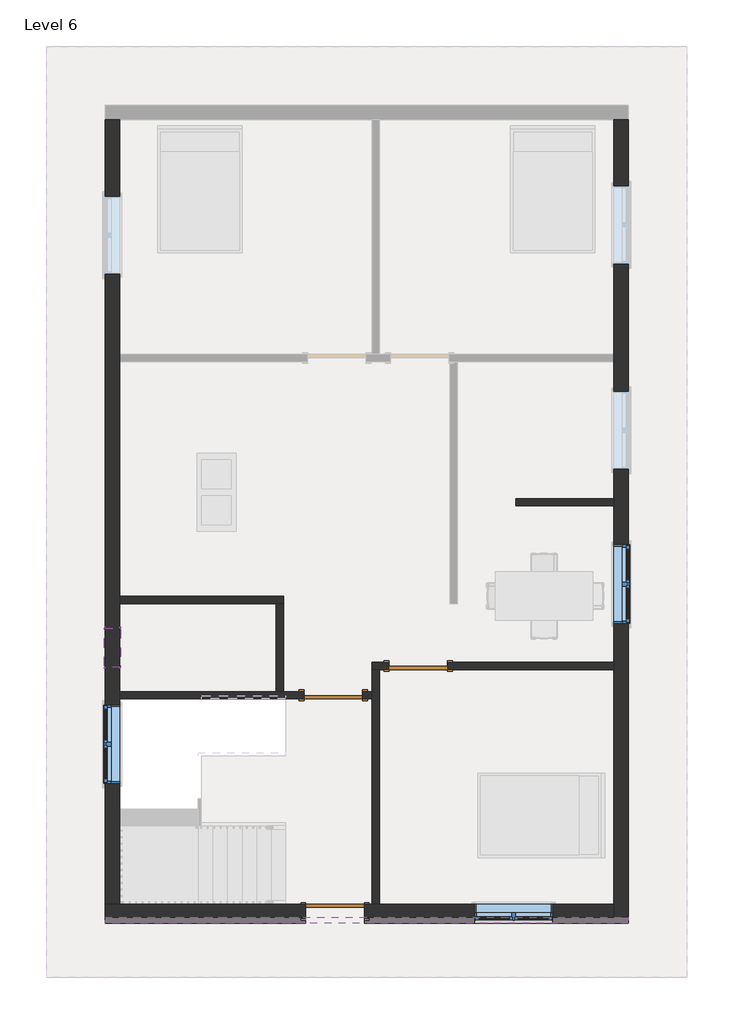
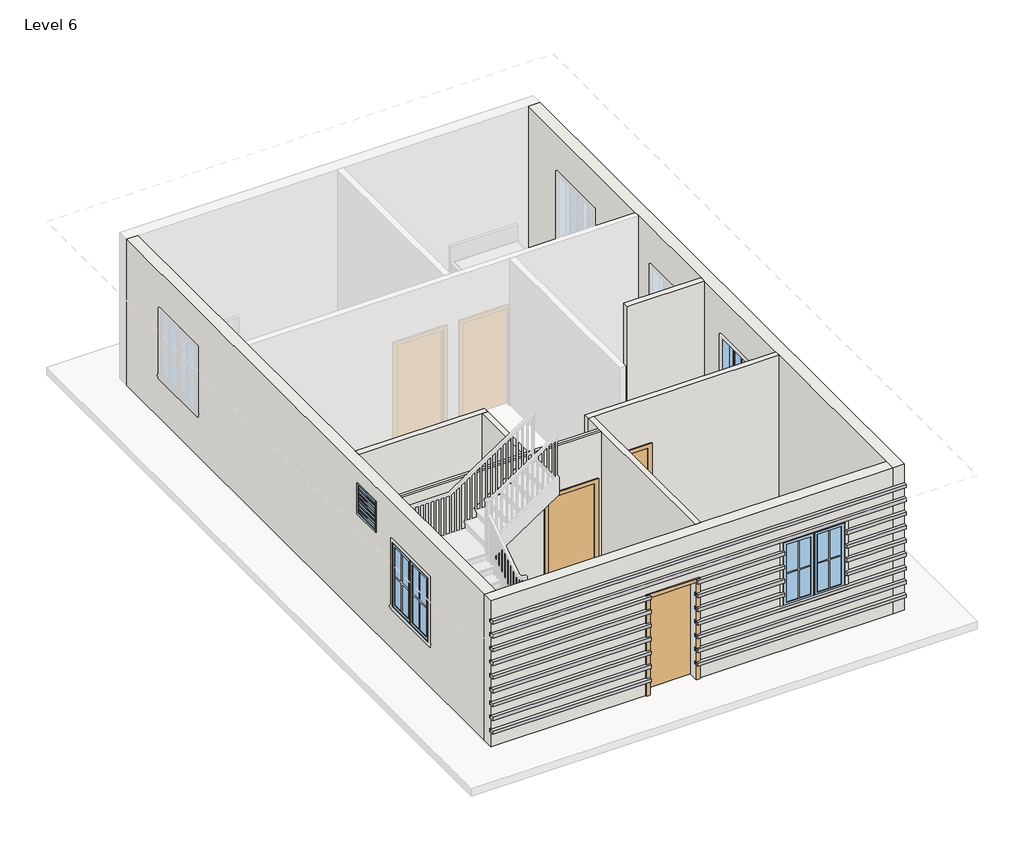
# One storey, part 1 of 3: 9 proxies, 9 walls, 4 windows, 3 doors.
"""IFC4 building model written with IfcOpenShell, lengths in millimetres."""

from ifc_helpers import new_model, si_unit, frame, origin, place, context, project, spatial, polyline, outline, extrude, faceted_brep, transform, mapped, element, save
from components import single_flush_door_3_17d80c48, single_flush_door_3_5e62189b, single_flush_door_3_89fc3733, window_casement_double_window_4_576b2d2c, window_f2d8fef0

model = new_model("IFC4")

# Units and contexts
model_context = context("Model", 3, world=origin())
ifc_project = project(units=[si_unit("LENGTHUNIT", "METRE", prefix="MILLI")], contexts=[model_context])

# Site, building, storey
site = spatial("IfcSite", under=ifc_project)
building = spatial("IfcBuilding", under=site)
storey = spatial("IfcBuildingStorey", under=building, Name="Level 6", Elevation=15849.6)

# Proxies
placement = place(None, origin())
element("IfcBuildingElementProxy", 1, Name="Reveal", ObjectType="Reveal", at=placement, inside=storey, context=model_context, shape_type="SweptSolid", body=[
    extrude(outline(polyline([(2831.4882597, -6585.4426559), (2831.4882597, -6677.5176559), (-1289.6617403, -6677.5176559), (-1289.6617403, -6585.4426559), (2831.4882597, -6585.4426559)])), frame((0.0, 0.0, 16154.4), z_axis=(0.0, 0.0, 1.0), x_axis=(1.0, 0.0, 0.0)), (0.0, 0.0, 1.0), 67.7333333),
    extrude(outline(polyline([(-2204.0617403, -6585.4426559), (-2204.0617403, -6677.5176559), (-5334.6117403, -6677.5176559), (-5334.6117403, -6585.4426559), (-2204.0617403, -6585.4426559)])), frame((0.0, 0.0, 16154.4), z_axis=(0.0, 0.0, 1.0), x_axis=(1.0, 0.0, 0.0)), (0.0, 0.0, 1.0), 67.7333333),
])
element("IfcBuildingElementProxy", 2, Name="Reveal", ObjectType="Reveal", at=placement, inside=storey, context=model_context, shape_type="SweptSolid", body=[
    extrude(outline(polyline([(2831.4882597, -6585.4426559), (2831.4882597, -6677.5176559), (-1289.6617403, -6677.5176559), (-1289.6617403, -6585.4426559), (2831.4882597, -6585.4426559)])), frame((0.0, 0.0, 16440.8994231), z_axis=(0.0, 0.0, 1.0), x_axis=(1.0, 0.0, 0.0)), (0.0, 0.0, 1.0), 67.7333333),
    extrude(outline(polyline([(-2204.0617403, -6585.4426559), (-2204.0617403, -6677.5176559), (-5334.6117403, -6677.5176559), (-5334.6117403, -6585.4426559), (-2204.0617403, -6585.4426559)])), frame((0.0, 0.0, 16440.8994231), z_axis=(0.0, 0.0, 1.0), x_axis=(1.0, 0.0, 0.0)), (0.0, 0.0, 1.0), 67.7333333),
])
element("IfcBuildingElementProxy", 3, Name="Reveal", ObjectType="Reveal", at=placement, inside=storey, context=model_context, shape_type="SweptSolid", body=[
    extrude(outline(polyline([(2831.4882597, -6585.4426559), (2831.4882597, -6677.5176559), (-1289.6617403, -6677.5176559), (-1289.6617403, -6585.4426559), (2831.4882597, -6585.4426559)])), frame((0.0, 0.0, 16727.3988461), z_axis=(0.0, 0.0, 1.0), x_axis=(1.0, 0.0, 0.0)), (0.0, 0.0, 1.0), 67.7333333),
    extrude(outline(polyline([(-2204.0617403, -6585.4426559), (-2204.0617403, -6677.5176559), (-5334.6117403, -6677.5176559), (-5334.6117403, -6585.4426559), (-2204.0617403, -6585.4426559)])), frame((0.0, 0.0, 16727.3988461), z_axis=(0.0, 0.0, 1.0), x_axis=(1.0, 0.0, 0.0)), (0.0, 0.0, 1.0), 67.7333333),
])
element("IfcBuildingElementProxy", 4, Name="Reveal", ObjectType="Reveal", at=placement, inside=storey, context=model_context, shape_type="SweptSolid", body=[
    extrude(outline(polyline([(2831.4882597, -6585.4426559), (2831.4882597, -6677.5176559), (1650.3882597, -6677.5176559), (1650.3882597, -6585.4426559), (2831.4882597, -6585.4426559)])), frame((0.0, 0.0, 17013.8982692), z_axis=(0.0, 0.0, 1.0), x_axis=(1.0, 0.0, 0.0)), (0.0, 0.0, 1.0), 67.7333333),
    extrude(outline(polyline([(431.1882597, -6585.4426559), (431.1882597, -6677.5176559), (-1289.6617403, -6677.5176559), (-1289.6617403, -6585.4426559), (431.1882597, -6585.4426559)])), frame((0.0, 0.0, 17013.8982692), z_axis=(0.0, 0.0, 1.0), x_axis=(1.0, 0.0, 0.0)), (0.0, 0.0, 1.0), 67.7333333),
    extrude(outline(polyline([(-2204.0617403, -6585.4426559), (-2204.0617403, -6677.5176559), (-5334.6117403, -6677.5176559), (-5334.6117403, -6585.4426559), (-2204.0617403, -6585.4426559)])), frame((0.0, 0.0, 17013.8982692), z_axis=(0.0, 0.0, 1.0), x_axis=(1.0, 0.0, 0.0)), (0.0, 0.0, 1.0), 67.7333333),
])
element("IfcBuildingElementProxy", 5, Name="Reveal", ObjectType="Reveal", at=placement, inside=storey, context=model_context, shape_type="SweptSolid", body=[
    extrude(outline(polyline([(2831.4882597, -6585.4426559), (2831.4882597, -6677.5176559), (1650.3882597, -6677.5176559), (1650.3882597, -6585.4426559), (2831.4882597, -6585.4426559)])), frame((0.0, 0.0, 17300.3976923), z_axis=(0.0, 0.0, 1.0), x_axis=(1.0, 0.0, 0.0)), (0.0, 0.0, 1.0), 67.7333333),
    extrude(outline(polyline([(431.1882597, -6585.4426559), (431.1882597, -6677.5176559), (-1289.6617403, -6677.5176559), (-1289.6617403, -6585.4426559), (431.1882597, -6585.4426559)])), frame((0.0, 0.0, 17300.3976923), z_axis=(0.0, 0.0, 1.0), x_axis=(1.0, 0.0, 0.0)), (0.0, 0.0, 1.0), 67.7333333),
    extrude(outline(polyline([(-2204.0617403, -6585.4426559), (-2204.0617403, -6677.5176559), (-5334.6117403, -6677.5176559), (-5334.6117403, -6585.4426559), (-2204.0617403, -6585.4426559)])), frame((0.0, 0.0, 17300.3976923), z_axis=(0.0, 0.0, 1.0), x_axis=(1.0, 0.0, 0.0)), (0.0, 0.0, 1.0), 67.7333333),
])
element("IfcBuildingElementProxy", 6, Name="Reveal", ObjectType="Reveal", at=placement, inside=storey, context=model_context, shape_type="SweptSolid", body=[
    extrude(outline(polyline([(2831.4882597, -6585.4426559), (2831.4882597, -6677.5176559), (1650.3882597, -6677.5176559), (1650.3882597, -6585.4426559), (2831.4882597, -6585.4426559)])), frame((0.0, 0.0, 17586.8971154), z_axis=(0.0, 0.0, 1.0), x_axis=(1.0, 0.0, 0.0)), (0.0, 0.0, 1.0), 67.7333333),
    extrude(outline(polyline([(431.1882597, -6585.4426559), (431.1882597, -6677.5176559), (-1289.6617403, -6677.5176559), (-1289.6617403, -6585.4426559), (431.1882597, -6585.4426559)])), frame((0.0, 0.0, 17586.8971154), z_axis=(0.0, 0.0, 1.0), x_axis=(1.0, 0.0, 0.0)), (0.0, 0.0, 1.0), 67.7333333),
    extrude(outline(polyline([(-2204.0617403, -6585.4426559), (-2204.0617403, -6677.5176559), (-5334.6117403, -6677.5176559), (-5334.6117403, -6585.4426559), (-2204.0617403, -6585.4426559)])), frame((0.0, 0.0, 17586.8971154), z_axis=(0.0, 0.0, 1.0), x_axis=(1.0, 0.0, 0.0)), (0.0, 0.0, 1.0), 67.7333333),
])
element("IfcBuildingElementProxy", 7, Name="Reveal", ObjectType="Reveal", at=placement, inside=storey, context=model_context, shape_type="SweptSolid", body=[
    extrude(outline(polyline([(2831.4882597, -6585.4426559), (2831.4882597, -6677.5176559), (1650.3882597, -6677.5176559), (1650.3882597, -6585.4426559), (2831.4882597, -6585.4426559)])), frame((0.0, 0.0, 17873.3965384), z_axis=(0.0, 0.0, 1.0), x_axis=(1.0, 0.0, 0.0)), (0.0, 0.0, 1.0), 67.7333333),
    extrude(outline(polyline([(431.1882597, -6585.4426559), (431.1882597, -6677.5176559), (-1289.6617403, -6677.5176559), (-1289.6617403, -6585.4426559), (431.1882597, -6585.4426559)])), frame((0.0, 0.0, 17873.3965384), z_axis=(0.0, 0.0, 1.0), x_axis=(1.0, 0.0, 0.0)), (0.0, 0.0, 1.0), 67.7333333),
    extrude(outline(polyline([(-2204.0617403, -6585.4426559), (-2204.0617403, -6677.5176559), (-5334.6117403, -6677.5176559), (-5334.6117403, -6585.4426559), (-2204.0617403, -6585.4426559)])), frame((0.0, 0.0, 17873.3965384), z_axis=(0.0, 0.0, 1.0), x_axis=(1.0, 0.0, 0.0)), (0.0, 0.0, 1.0), 67.7333333),
])
element("IfcBuildingElementProxy", 8, Name="Reveal", ObjectType="Reveal", at=placement, inside=storey, context=model_context, shape_type="SweptSolid", body=[
    extrude(outline(polyline([(2831.4882597, -6585.4426559), (2831.4882597, -6677.5176559), (-5334.6117403, -6677.5176559), (-5334.6117403, -6585.4426559), (2831.4882597, -6585.4426559)])), frame((0.0, 0.0, 18159.8959615), z_axis=(0.0, 0.0, 1.0), x_axis=(1.0, 0.0, 0.0)), (0.0, 0.0, 1.0), 67.7333333),
])
element("IfcBuildingElementProxy", 9, Name="Reveal", ObjectType="Reveal", at=placement, inside=storey, context=model_context, shape_type="SweptSolid", body=[
    extrude(outline(polyline([(2831.4882597, -6585.4426559), (2831.4882597, -6677.5176559), (-5334.6117403, -6677.5176559), (-5334.6117403, -6585.4426559), (2831.4882597, -6585.4426559)])), frame((0.0, 0.0, 18446.3953846), z_axis=(0.0, 0.0, 1.0), x_axis=(1.0, 0.0, 0.0)), (0.0, 0.0, 1.0), 67.7333333),
])

# Doors
single_flush_door_3_shape = single_flush_door_3_17d80c48(model_context)
element("IfcDoor", 10, ObjectType="Single-Flush : DOOR 3'", at=placement, inside=storey, context=model_context, shape_type="MappedRepresentation", body=[
    mapped(single_flush_door_3_shape, transform((-451.4617403, -2667.4926559, 15849.6), x_axis=(-1.0, 0.0, 0.0), y_axis=(0.0, -1.0, 0.0), z_axis=(0.0, 0.0, 1.0))),
])
single_flush_door_3_2_shape = single_flush_door_3_5e62189b(model_context)
element("IfcDoor", 11, ObjectType="Single-Flush : DOOR 3'", at=placement, inside=storey, context=model_context, shape_type="MappedRepresentation", body=[
    mapped(single_flush_door_3_2_shape, transform((-1772.2617403, -3124.6926559, 15849.6), x_axis=(1.0, 0.0, 0.0), y_axis=(0.0, 1.0, 0.0), z_axis=(0.0, 0.0, 1.0))),
])
single_flush_door_3_3_shape = single_flush_door_3_89fc3733(model_context)
element("IfcDoor", 12, ObjectType="Single-Flush : DOOR 3'", at=placement, inside=storey, context=model_context, shape_type="MappedRepresentation", body=[
    mapped(single_flush_door_3_3_shape, transform((-1746.8617403, -6496.5426559, 15849.6), x_axis=(1.0, 0.0, 0.0), y_axis=(0.0, 1.0, 0.0), z_axis=(0.0, 0.0, 1.0))),
])

# Walls
element("IfcWall", 13, ObjectType="ALL 4.5\"", at=placement, inside=storey, context=model_context, shape_type="SweptSolid", body=[
    extrude(outline(polyline([(1078.8882597, -57.6426559), (2602.8882597, -57.6426559), (2602.8882597, -171.9426559), (1078.8882597, -171.9426559), (1078.8882597, -57.6426559)])), frame((0.0, 0.0, 15849.6), z_axis=(0.0, 0.0, 1.0), x_axis=(1.0, 0.0, 0.0)), (0.0, 0.0, 1.0), 3048.0),
])
element("IfcWall", 14, ObjectType="ALL 4.5\"", at=placement, inside=storey, context=model_context, shape_type="Brep", body=[
    faceted_brep([(-908.6617403, -2610.3426559, 17881.6), (-908.6617403, -2610.3426559, 15849.6), (-1169.0117403, -2610.3426559, 15849.6), (-1169.0117403, -2610.3426559, 18897.6), (2602.8882597, -2610.3426559, 18897.6), (2602.8882597, -2610.3426559, 15849.6), (5.7382597, -2610.3426559, 15849.6), (5.7382597, -2610.3426559, 17881.6), (-1169.0117403, -2724.6426559, 15849.6), (-1054.7117403, -2724.6426559, 15849.6), (-908.6617403, -2724.6426559, 15849.6), (-908.6617403, -2724.6426559, 17881.6), (5.7382597, -2724.6426559, 17881.6), (5.7382597, -2724.6426559, 15849.6), (2602.8882597, -2724.6426559, 15849.6), (2602.8882597, -2724.6426559, 18897.6), (-1054.7117403, -2724.6426559, 18897.6), (-1169.0117403, -2724.6426559, 18897.6)], [[[0, 1, 2, 3, 4, 5, 6, 7]], [[8, 9, 10, 11, 12, 13, 14, 15, 16, 17]], [[6, 5, 14, 13]], [[2, 1, 10, 9, 8]], [[5, 4, 15, 14]], [[3, 2, 8, 17]], [[11, 10, 1, 0]], [[12, 11, 0, 7]], [[13, 12, 7, 6]], [[4, 3, 17, 16, 15]]]),
])
element("IfcWall", 15, ObjectType="ALL 4.5\"", at=placement, inside=storey, context=model_context, shape_type="Brep", body=[
    faceted_brep([(-1169.0117403, -2724.6426559, 15849.6), (-1169.0117403, -3067.5426559, 15849.6), (-1169.0117403, -3181.8426559, 15849.6), (-1169.0117403, -6382.2426559, 15849.6), (-1169.0117403, -6382.2426559, 18897.6), (-1169.0117403, -3181.8426559, 18897.6), (-1169.0117403, -3067.5426559, 18897.6), (-1169.0117403, -2724.6426559, 18897.6), (-1054.7117403, -2724.6426559, 15849.6), (-1054.7117403, -2724.6426559, 18897.6), (-1054.7117403, -6382.2426559, 18897.6), (-1054.7117403, -6382.2426559, 15849.6)], [[[0, 1, 2, 3, 4, 5, 6, 7]], [[8, 9, 10, 11]], [[3, 2, 1, 0, 8, 11]], [[0, 7, 9, 8]], [[4, 3, 11, 10]], [[7, 6, 5, 4, 10, 9]]]),
])
element("IfcWall", 16, ObjectType="ALL 4.5\"", at=placement, inside=storey, context=model_context, shape_type="Brep", body=[
    faceted_brep([(-1169.0117403, -3067.5426559, 15849.6), (-1315.0617403, -3067.5426559, 15849.6), (-1315.0617403, -3067.5426559, 17881.6), (-2229.4617403, -3067.5426559, 17881.6), (-2229.4617403, -3067.5426559, 15849.6), (-2553.3117403, -3067.5426559, 15849.6), (-2667.6117403, -3067.5426559, 15849.6), (-5106.0117403, -3067.5426559, 15849.6), (-5106.0117403, -3067.5426559, 18897.6), (-2667.6117403, -3067.5426559, 18897.6), (-2553.3117403, -3067.5426559, 18897.6), (-1169.0117403, -3067.5426559, 18897.6), (-1315.0617403, -3181.8426559, 17881.6), (-1315.0617403, -3181.8426559, 15849.6), (-1169.0117403, -3181.8426559, 15849.6), (-1169.0117403, -3181.8426559, 18897.6), (-5106.0117403, -3181.8426559, 18897.6), (-5106.0117403, -3181.8426559, 15849.6), (-2229.4617403, -3181.8426559, 15849.6), (-2229.4617403, -3181.8426559, 17881.6), (-5106.0117403, -3131.0426559, 18897.6), (-1169.0117403, -3131.0426559, 18897.6), (-2515.2117403, -3131.0426559, 18897.6)], [[[0, 1, 2, 3, 4, 5, 6, 7, 8, 9, 10, 11]], [[12, 13, 14, 15, 16, 17, 18, 19]], [[18, 17, 7, 6, 5, 4]], [[14, 13, 1, 0]], [[8, 7, 17, 16, 20]], [[0, 11, 21, 15, 14]], [[2, 1, 13, 12]], [[3, 2, 12, 19]], [[4, 3, 19, 18]], [[11, 10, 9, 8, 20, 22, 21]], [[20, 16, 15, 21, 22]]]),
])
element("IfcWall", 17, ObjectType="ALL 4.5\"", at=placement, inside=storey, context=model_context, shape_type="Brep", body=[
    faceted_brep([(-5106.0117403, -1695.9426559, 15849.6), (-2667.6117403, -1695.9426559, 15849.6), (-2553.3117403, -1695.9426559, 15849.6), (-2553.3117403, -1695.9426559, 18897.6), (-2667.6117403, -1695.9426559, 18897.6), (-5106.0117403, -1695.9426559, 18897.6), (-5106.0117403, -1581.6426559, 15849.6), (-5106.0117403, -1581.6426559, 18897.6), (-2553.3117403, -1581.6426559, 18897.6), (-2553.3117403, -1581.6426559, 15849.6)], [[[0, 1, 2, 3, 4, 5]], [[6, 7, 8, 9]], [[2, 1, 0, 6, 9]], [[0, 5, 7, 6]], [[3, 2, 9, 8]], [[5, 4, 3, 8, 7]]]),
])
element("IfcWall", 18, ObjectType="ALL 4.5\"", at=placement, inside=storey, context=model_context, shape_type="SweptSolid", body=[
    extrude(outline(polyline([(-2667.6117403, -3067.5426559), (-2667.6117403, -1695.9426559), (-2553.3117403, -1695.9426559), (-2553.3117403, -3067.5426559), (-2667.6117403, -3067.5426559)])), frame((0.0, 0.0, 15849.6), z_axis=(0.0, 0.0, 1.0), x_axis=(1.0, 0.0, 0.0)), (0.0, 0.0, 1.0), 3048.0),
])
element("IfcWall", 19, ObjectType="WALL 9\"", at=placement, inside=storey, context=model_context, shape_type="Brep", body=[
    faceted_brep([(2602.8882597, 5847.8573441, 15849.6), (2602.8882597, 2190.2573441, 15849.6), (2602.8882597, 2075.9573441, 15849.6), (2602.8882597, -57.6426559, 15849.6), (2602.8882597, -171.9426559, 15849.6), (2602.8882597, -2610.3426559, 15849.6), (2602.8882597, -2724.6426559, 15849.6), (2602.8882597, -6382.2426559, 15849.6), (2602.8882597, -6610.8426559, 15849.6), (2602.8882597, -6610.8426559, 16154.4), (2602.8882597, -6585.4426559, 16154.4), (2602.8882597, -6585.4426559, 16222.1333333), (2602.8882597, -6610.8426559, 16222.1333333), (2602.8882597, -6610.8426559, 16440.8994231), (2602.8882597, -6585.4426559, 16440.8994231), (2602.8882597, -6585.4426559, 16508.6327564), (2602.8882597, -6610.8426559, 16508.6327564), (2602.8882597, -6610.8426559, 16727.3988461), (2602.8882597, -6585.4426559, 16727.3988461), (2602.8882597, -6585.4426559, 16795.1321795), (2602.8882597, -6610.8426559, 16795.1321795), (2602.8882597, -6610.8426559, 17013.8982692), (2602.8882597, -6585.4426559, 17013.8982692), (2602.8882597, -6585.4426559, 17081.6316025), (2602.8882597, -6610.8426559, 17081.6316025), (2602.8882597, -6610.8426559, 17300.3976923), (2602.8882597, -6585.4426559, 17300.3976923), (2602.8882597, -6585.4426559, 17368.1310256), (2602.8882597, -6610.8426559, 17368.1310256), (2602.8882597, -6610.8426559, 17586.8971154), (2602.8882597, -6585.4426559, 17586.8971154), (2602.8882597, -6585.4426559, 17654.6304487), (2602.8882597, -6610.8426559, 17654.6304487), (2602.8882597, -6610.8426559, 17873.3965384), (2602.8882597, -6585.4426559, 17873.3965384), (2602.8882597, -6585.4426559, 17941.1298718), (2602.8882597, -6610.8426559, 17941.1298718), (2602.8882597, -6610.8426559, 18159.8959615), (2602.8882597, -6585.4426559, 18159.8959615), (2602.8882597, -6585.4426559, 18227.6292948), (2602.8882597, -6610.8426559, 18227.6292948), (2602.8882597, -6610.8426559, 18446.3953846), (2602.8882597, -6585.4426559, 18446.3953846), (2602.8882597, -6585.4426559, 18514.1287179), (2602.8882597, -6610.8426559, 18514.1287179), (2602.8882597, -6610.8426559, 18897.6), (2602.8882597, -6382.2426559, 18897.6), (2602.8882597, -2724.6426559, 18897.6), (2602.8882597, -2610.3426559, 18897.6), (2602.8882597, -171.9426559, 18897.6), (2602.8882597, -57.6426559, 18897.6), (2602.8882597, 2075.9573441, 18897.6), (2602.8882597, 2190.2573441, 18897.6), (2602.8882597, 5847.8573441, 18897.6), (2602.8882597, 3599.9573441, 18110.2), (2602.8882597, 3599.9573441, 16764.0), (2602.8882597, 4819.1573441, 16764.0), (2602.8882597, 4819.1573441, 18110.2), (2602.8882597, 399.5573441, 18110.2), (2602.8882597, 399.5573441, 16764.0), (2602.8882597, 1618.7573441, 16764.0), (2602.8882597, 1618.7573441, 18110.2), (2602.8882597, -2000.7426559, 18110.2), (2602.8882597, -2000.7426559, 16764.0), (2602.8882597, -781.5426559, 16764.0), (2602.8882597, -781.5426559, 18110.2), (2831.4882597, -6610.8426559, 15849.6), (2831.4882597, 5847.8573441, 15849.6), (2831.4882597, 5847.8573441, 18897.6), (2831.4882597, -6610.8426559, 18897.6), (2831.4882597, -6610.8426559, 18514.1287179), (2831.4882597, -6585.4426559, 18514.1287179), (2831.4882597, -6585.4426559, 18446.3953846), (2831.4882597, -6610.8426559, 18446.3953846), (2831.4882597, -6610.8426559, 18227.6292948), (2831.4882597, -6585.4426559, 18227.6292948), (2831.4882597, -6585.4426559, 18159.8959615), (2831.4882597, -6610.8426559, 18159.8959615), (2831.4882597, -6610.8426559, 17941.1298718), (2831.4882597, -6585.4426559, 17941.1298718), (2831.4882597, -6585.4426559, 17873.3965384), (2831.4882597, -6610.8426559, 17873.3965384), (2831.4882597, -6610.8426559, 17654.6304487), (2831.4882597, -6585.4426559, 17654.6304487), (2831.4882597, -6585.4426559, 17586.8971154), (2831.4882597, -6610.8426559, 17586.8971154), (2831.4882597, -6610.8426559, 17368.1310256), (2831.4882597, -6585.4426559, 17368.1310256), (2831.4882597, -6585.4426559, 17300.3976923), (2831.4882597, -6610.8426559, 17300.3976923), (2831.4882597, -6610.8426559, 17081.6316025), (2831.4882597, -6585.4426559, 17081.6316025), (2831.4882597, -6585.4426559, 17013.8982692), (2831.4882597, -6610.8426559, 17013.8982692), (2831.4882597, -6610.8426559, 16795.1321795), (2831.4882597, -6585.4426559, 16795.1321795), (2831.4882597, -6585.4426559, 16727.3988461), (2831.4882597, -6610.8426559, 16727.3988461), (2831.4882597, -6610.8426559, 16508.6327564), (2831.4882597, -6585.4426559, 16508.6327564), (2831.4882597, -6585.4426559, 16440.8994231), (2831.4882597, -6610.8426559, 16440.8994231), (2831.4882597, -6610.8426559, 16222.1333333), (2831.4882597, -6585.4426559, 16222.1333333), (2831.4882597, -6585.4426559, 16154.4), (2831.4882597, -6610.8426559, 16154.4), (2831.4882597, 3599.9573441, 16764.0), (2831.4882597, 3599.9573441, 18110.2), (2831.4882597, 4819.1573441, 18110.2), (2831.4882597, 4819.1573441, 16764.0), (2831.4882597, 399.5573441, 16764.0), (2831.4882597, 399.5573441, 18110.2), (2831.4882597, 1618.7573441, 18110.2), (2831.4882597, 1618.7573441, 16764.0), (2831.4882597, -2000.7426559, 16764.0), (2831.4882597, -2000.7426559, 18110.2), (2831.4882597, -781.5426559, 18110.2), (2831.4882597, -781.5426559, 16764.0)], [[[0, 1, 2, 3, 4, 5, 6, 7, 8, 9, 10, 11, 12, 13, 14, 15, 16, 17, 18, 19, 20, 21, 22, 23, 24, 25, 26, 27, 28, 29, 30, 31, 32, 33, 34, 35, 36, 37, 38, 39, 40, 41, 42, 43, 44, 45, 46, 47, 48, 49, 50, 51, 52, 53], [54, 55, 56, 57], [58, 59, 60, 61], [62, 63, 64, 65]], [[66, 67, 68, 69, 70, 71, 72, 73, 74, 75, 76, 77, 78, 79, 80, 81, 82, 83, 84, 85, 86, 87, 88, 89, 90, 91, 92, 93, 94, 95, 96, 97, 98, 99, 100, 101, 102, 103, 104, 105], [106, 107, 108, 109], [110, 111, 112, 113], [114, 115, 116, 117]], [[8, 7, 6, 5, 4, 3, 2, 1, 0, 67, 66]], [[0, 53, 68, 67]], [[8, 66, 105, 9]], [[69, 45, 44, 70]], [[12, 102, 101, 13]], [[16, 98, 97, 17]], [[20, 94, 93, 21]], [[24, 90, 89, 25]], [[28, 86, 85, 29]], [[32, 82, 81, 33]], [[36, 78, 77, 37]], [[40, 74, 73, 41]], [[55, 54, 107, 106]], [[56, 55, 106, 109]], [[57, 56, 109, 108]], [[54, 57, 108, 107]], [[59, 58, 111, 110]], [[60, 59, 110, 113]], [[61, 60, 113, 112]], [[58, 61, 112, 111]], [[63, 62, 115, 114]], [[64, 63, 114, 117]], [[65, 64, 117, 116]], [[62, 65, 116, 115]], [[53, 52, 51, 50, 49, 48, 47, 46, 45, 69, 68]], [[11, 103, 102, 12]], [[104, 10, 9, 105]], [[103, 11, 10, 104]], [[15, 99, 98, 16]], [[100, 14, 13, 101]], [[99, 15, 14, 100]], [[19, 95, 94, 20]], [[96, 18, 17, 97]], [[95, 19, 18, 96]], [[23, 91, 90, 24]], [[92, 22, 21, 93]], [[91, 23, 22, 92]], [[27, 87, 86, 28]], [[88, 26, 25, 89]], [[87, 27, 26, 88]], [[31, 83, 82, 32]], [[84, 30, 29, 85]], [[83, 31, 30, 84]], [[35, 79, 78, 36]], [[80, 34, 33, 81]], [[79, 35, 34, 80]], [[39, 75, 74, 40]], [[76, 38, 37, 77]], [[75, 39, 38, 76]], [[43, 71, 70, 44]], [[72, 42, 41, 73]], [[71, 43, 42, 72]]]),
])
element("IfcWall", 20, ObjectType="WALL 9\"", at=placement, inside=storey, context=model_context, shape_type="Brep", body=[
    faceted_brep([(-5334.6117403, -6382.2426559, 18897.6), (-5106.0117403, -6382.2426559, 18897.6), (-1169.0117403, -6382.2426559, 18897.6), (-1054.7117403, -6382.2426559, 18897.6), (2602.8882597, -6382.2426559, 18897.6), (2602.8882597, -6382.2426559, 15849.6), (-1054.7117403, -6382.2426559, 15849.6), (-1169.0117403, -6382.2426559, 15849.6), (-1289.6617403, -6382.2426559, 15849.6), (-1289.6617403, -6382.2426559, 17881.6), (-2204.0617403, -6382.2426559, 17881.6), (-2204.0617403, -6382.2426559, 15849.6), (-5106.0117403, -6382.2426559, 15849.6), (-5334.6117403, -6382.2426559, 15849.6), (431.1882597, -6382.2426559, 18110.2), (431.1882597, -6382.2426559, 16764.0), (1650.3882597, -6382.2426559, 16764.0), (1650.3882597, -6382.2426559, 18110.2), (2602.8882597, -6610.8426559, 18897.6), (-5334.6117403, -6610.8426559, 18897.6), (-5334.6117403, -6610.8426559, 18514.1287179), (2602.8882597, -6610.8426559, 18514.1287179), (431.1882597, -6610.8426559, 18110.2), (1650.3882597, -6610.8426559, 18110.2), (1650.3882597, -6610.8426559, 17941.1298718), (2602.8882597, -6610.8426559, 17941.1298718), (2602.8882597, -6610.8426559, 18159.8959615), (-5334.6117403, -6610.8426559, 18159.8959615), (-5334.6117403, -6610.8426559, 17941.1298718), (-2204.0617403, -6610.8426559, 17941.1298718), (-2204.0617403, -6610.8426559, 17881.6), (-1289.6617403, -6610.8426559, 17881.6), (-1289.6617403, -6610.8426559, 17941.1298718), (431.1882597, -6610.8426559, 17941.1298718), (-5334.6117403, -6610.8426559, 15849.6), (-2204.0617403, -6610.8426559, 15849.6), (-2204.0617403, -6610.8426559, 16154.4), (-5334.6117403, -6610.8426559, 16154.4), (-1289.6617403, -6610.8426559, 15849.6), (2602.8882597, -6610.8426559, 15849.6), (2602.8882597, -6610.8426559, 16154.4), (-1289.6617403, -6610.8426559, 16154.4), (-1289.6617403, -6610.8426559, 16222.1333333), (2602.8882597, -6610.8426559, 16222.1333333), (2602.8882597, -6610.8426559, 16440.8994231), (-1289.6617403, -6610.8426559, 16440.8994231), (-5334.6117403, -6610.8426559, 16222.1333333), (-2204.0617403, -6610.8426559, 16222.1333333), (-2204.0617403, -6610.8426559, 16440.8994231), (-5334.6117403, -6610.8426559, 16440.8994231), (-1289.6617403, -6610.8426559, 16508.6327564), (2602.8882597, -6610.8426559, 16508.6327564), (2602.8882597, -6610.8426559, 16727.3988461), (-1289.6617403, -6610.8426559, 16727.3988461), (-5334.6117403, -6610.8426559, 16508.6327564), (-2204.0617403, -6610.8426559, 16508.6327564), (-2204.0617403, -6610.8426559, 16727.3988461), (-5334.6117403, -6610.8426559, 16727.3988461), (-1289.6617403, -6610.8426559, 16795.1321795), (431.1882597, -6610.8426559, 16795.1321795), (431.1882597, -6610.8426559, 17013.8982692), (-1289.6617403, -6610.8426559, 17013.8982692), (1650.3882597, -6610.8426559, 16795.1321795), (2602.8882597, -6610.8426559, 16795.1321795), (2602.8882597, -6610.8426559, 17013.8982692), (1650.3882597, -6610.8426559, 17013.8982692), (-5334.6117403, -6610.8426559, 16795.1321795), (-2204.0617403, -6610.8426559, 16795.1321795), (-2204.0617403, -6610.8426559, 17013.8982692), (-5334.6117403, -6610.8426559, 17013.8982692), (1650.3882597, -6610.8426559, 17081.6316025), (2602.8882597, -6610.8426559, 17081.6316025), (2602.8882597, -6610.8426559, 17300.3976923), (1650.3882597, -6610.8426559, 17300.3976923), (-1289.6617403, -6610.8426559, 17081.6316025), (431.1882597, -6610.8426559, 17081.6316025), (431.1882597, -6610.8426559, 17300.3976923), (-1289.6617403, -6610.8426559, 17300.3976923), (-5334.6117403, -6610.8426559, 17081.6316025), (-2204.0617403, -6610.8426559, 17081.6316025), (-2204.0617403, -6610.8426559, 17300.3976923), (-5334.6117403, -6610.8426559, 17300.3976923), (1650.3882597, -6610.8426559, 17368.1310256), (2602.8882597, -6610.8426559, 17368.1310256), (2602.8882597, -6610.8426559, 17586.8971154), (1650.3882597, -6610.8426559, 17586.8971154), (-1289.6617403, -6610.8426559, 17368.1310256), (431.1882597, -6610.8426559, 17368.1310256), (431.1882597, -6610.8426559, 17586.8971154), (-1289.6617403, -6610.8426559, 17586.8971154), (-5334.6117403, -6610.8426559, 17368.1310256), (-2204.0617403, -6610.8426559, 17368.1310256), (-2204.0617403, -6610.8426559, 17586.8971154), (-5334.6117403, -6610.8426559, 17586.8971154), (1650.3882597, -6610.8426559, 17654.6304487), (2602.8882597, -6610.8426559, 17654.6304487), (2602.8882597, -6610.8426559, 17873.3965384), (1650.3882597, -6610.8426559, 17873.3965384), (-1289.6617403, -6610.8426559, 17654.6304487), (431.1882597, -6610.8426559, 17654.6304487), (431.1882597, -6610.8426559, 17873.3965384), (-1289.6617403, -6610.8426559, 17873.3965384), (-5334.6117403, -6610.8426559, 17654.6304487), (-2204.0617403, -6610.8426559, 17654.6304487), (-2204.0617403, -6610.8426559, 17873.3965384), (-5334.6117403, -6610.8426559, 17873.3965384), (-5334.6117403, -6610.8426559, 18227.6292948), (2602.8882597, -6610.8426559, 18227.6292948), (2602.8882597, -6610.8426559, 18446.3953846), (-5334.6117403, -6610.8426559, 18446.3953846), (2602.8882597, -6585.4426559, 18514.1287179), (2602.8882597, -6585.4426559, 18446.3953846), (2602.8882597, -6585.4426559, 18227.6292948), (2602.8882597, -6585.4426559, 18159.8959615), (2602.8882597, -6585.4426559, 17941.1298718), (2602.8882597, -6585.4426559, 17873.3965384), (2602.8882597, -6585.4426559, 17654.6304487), (2602.8882597, -6585.4426559, 17586.8971154), (2602.8882597, -6585.4426559, 17368.1310256), (2602.8882597, -6585.4426559, 17300.3976923), (2602.8882597, -6585.4426559, 17081.6316025), (2602.8882597, -6585.4426559, 17013.8982692), (2602.8882597, -6585.4426559, 16795.1321795), (2602.8882597, -6585.4426559, 16727.3988461), (2602.8882597, -6585.4426559, 16508.6327564), (2602.8882597, -6585.4426559, 16440.8994231), (2602.8882597, -6585.4426559, 16222.1333333), (2602.8882597, -6585.4426559, 16154.4), (-5334.6117403, -6585.4426559, 16154.4), (-5334.6117403, -6585.4426559, 16222.1333333), (-5334.6117403, -6585.4426559, 16440.8994231), (-5334.6117403, -6585.4426559, 16508.6327564), (-5334.6117403, -6585.4426559, 16727.3988461), (-5334.6117403, -6585.4426559, 16795.1321795), (-5334.6117403, -6585.4426559, 17013.8982692), (-5334.6117403, -6585.4426559, 17081.6316025), (-5334.6117403, -6585.4426559, 17300.3976923), (-5334.6117403, -6585.4426559, 17368.1310256), (-5334.6117403, -6585.4426559, 17586.8971154), (-5334.6117403, -6585.4426559, 17654.6304487), (-5334.6117403, -6585.4426559, 17873.3965384), (-5334.6117403, -6585.4426559, 17941.1298718), (-5334.6117403, -6585.4426559, 18159.8959615), (-5334.6117403, -6585.4426559, 18227.6292948), (-5334.6117403, -6585.4426559, 18446.3953846), (-5334.6117403, -6585.4426559, 18514.1287179), (431.1882597, -6585.4426559, 17941.1298718), (431.1882597, -6585.4426559, 17873.3965384), (431.1882597, -6585.4426559, 17654.6304487), (431.1882597, -6585.4426559, 17586.8971154), (431.1882597, -6585.4426559, 17368.1310256), (431.1882597, -6585.4426559, 17300.3976923), (431.1882597, -6585.4426559, 17081.6316025), (431.1882597, -6585.4426559, 17013.8982692), (431.1882597, -6585.4426559, 16795.1321795), (431.1882597, -6585.4426559, 16764.0), (1650.3882597, -6585.4426559, 16764.0), (1650.3882597, -6585.4426559, 16795.1321795), (1650.3882597, -6585.4426559, 17013.8982692), (1650.3882597, -6585.4426559, 17081.6316025), (1650.3882597, -6585.4426559, 17300.3976923), (1650.3882597, -6585.4426559, 17368.1310256), (1650.3882597, -6585.4426559, 17586.8971154), (1650.3882597, -6585.4426559, 17654.6304487), (1650.3882597, -6585.4426559, 17873.3965384), (1650.3882597, -6585.4426559, 17941.1298718), (-1289.6617403, -6585.4426559, 16154.4), (-1289.6617403, -6585.4426559, 16222.1333333), (-1289.6617403, -6585.4426559, 16440.8994231), (-1289.6617403, -6585.4426559, 16508.6327564), (-1289.6617403, -6585.4426559, 16727.3988461), (-1289.6617403, -6585.4426559, 16795.1321795), (-1289.6617403, -6585.4426559, 17013.8982692), (-1289.6617403, -6585.4426559, 17081.6316025), (-1289.6617403, -6585.4426559, 17300.3976923), (-1289.6617403, -6585.4426559, 17368.1310256), (-1289.6617403, -6585.4426559, 17586.8971154), (-1289.6617403, -6585.4426559, 17654.6304487), (-1289.6617403, -6585.4426559, 17873.3965384), (-1289.6617403, -6585.4426559, 17881.6), (-2204.0617403, -6585.4426559, 17881.6), (-2204.0617403, -6585.4426559, 17873.3965384), (-2204.0617403, -6585.4426559, 17654.6304487), (-2204.0617403, -6585.4426559, 17586.8971154), (-2204.0617403, -6585.4426559, 17368.1310256), (-2204.0617403, -6585.4426559, 17300.3976923), (-2204.0617403, -6585.4426559, 17081.6316025), (-2204.0617403, -6585.4426559, 17013.8982692), (-2204.0617403, -6585.4426559, 16795.1321795), (-2204.0617403, -6585.4426559, 16727.3988461), (-2204.0617403, -6585.4426559, 16508.6327564), (-2204.0617403, -6585.4426559, 16440.8994231), (-2204.0617403, -6585.4426559, 16222.1333333), (-2204.0617403, -6585.4426559, 16154.4), (-1289.6617403, -6585.4426559, 17941.1298718), (-2204.0617403, -6585.4426559, 17941.1298718)], [[[0, 1, 2, 3, 4, 5, 6, 7, 8, 9, 10, 11, 12, 13], [14, 15, 16, 17]], [[18, 19, 20, 21]], [[22, 23, 24, 25, 26, 27, 28, 29, 30, 31, 32, 33]], [[34, 35, 36, 37]], [[38, 39, 40, 41]], [[42, 43, 44, 45]], [[46, 47, 48, 49]], [[50, 51, 52, 53]], [[54, 55, 56, 57]], [[58, 59, 60, 61]], [[62, 63, 64, 65]], [[66, 67, 68, 69]], [[70, 71, 72, 73]], [[74, 75, 76, 77]], [[78, 79, 80, 81]], [[82, 83, 84, 85]], [[86, 87, 88, 89]], [[90, 91, 92, 93]], [[94, 95, 96, 97]], [[98, 99, 100, 101]], [[102, 103, 104, 105]], [[106, 107, 108, 109]], [[5, 39, 38, 8, 7, 6]], [[34, 13, 12, 11, 35]], [[4, 3, 2, 1, 0, 19, 18]], [[5, 4, 18, 21, 110, 111, 108, 107, 112, 113, 26, 25, 114, 115, 96, 95, 116, 117, 84, 83, 118, 119, 72, 71, 120, 121, 64, 63, 122, 123, 52, 51, 124, 125, 44, 43, 126, 127, 40, 39]], [[0, 13, 34, 37, 128, 129, 46, 49, 130, 131, 54, 57, 132, 133, 66, 69, 134, 135, 78, 81, 136, 137, 90, 93, 138, 139, 102, 105, 140, 141, 28, 27, 142, 143, 106, 109, 144, 145, 20, 19]], [[15, 14, 22, 33, 146, 147, 100, 99, 148, 149, 88, 87, 150, 151, 76, 75, 152, 153, 60, 59, 154, 155]], [[16, 15, 155, 156]], [[17, 16, 156, 157, 62, 65, 158, 159, 70, 73, 160, 161, 82, 85, 162, 163, 94, 97, 164, 165, 24, 23]], [[14, 17, 23, 22]], [[9, 8, 38, 41, 166, 167, 42, 45, 168, 169, 50, 53, 170, 171, 58, 61, 172, 173, 74, 77, 174, 175, 86, 89, 176, 177, 98, 101, 178, 179]], [[10, 9, 179, 31, 30, 180]], [[11, 10, 180, 181, 104, 103, 182, 183, 92, 91, 184, 185, 80, 79, 186, 187, 68, 67, 188, 189, 56, 55, 190, 191, 48, 47, 192, 193, 36, 35]], [[167, 126, 43, 42]], [[127, 166, 41, 40]], [[126, 167, 166, 127]], [[129, 192, 47, 46]], [[193, 128, 37, 36]], [[192, 129, 128, 193]], [[169, 124, 51, 50]], [[125, 168, 45, 44]], [[124, 169, 168, 125]], [[131, 190, 55, 54]], [[191, 130, 49, 48]], [[190, 131, 130, 191]], [[171, 154, 59, 58]], [[157, 122, 63, 62]], [[123, 170, 53, 52]], [[154, 171, 170, 123, 122, 157, 156, 155]], [[133, 188, 67, 66]], [[189, 132, 57, 56]], [[188, 133, 132, 189]], [[159, 120, 71, 70]], [[121, 158, 65, 64]], [[120, 159, 158, 121]], [[173, 152, 75, 74]], [[153, 172, 61, 60]], [[152, 173, 172, 153]], [[135, 186, 79, 78]], [[187, 134, 69, 68]], [[186, 135, 134, 187]], [[161, 118, 83, 82]], [[119, 160, 73, 72]], [[118, 161, 160, 119]], [[175, 150, 87, 86]], [[151, 174, 77, 76]], [[150, 175, 174, 151]], [[137, 184, 91, 90]], [[185, 136, 81, 80]], [[184, 137, 136, 185]], [[163, 116, 95, 94]], [[117, 162, 85, 84]], [[116, 163, 162, 117]], [[177, 148, 99, 98]], [[149, 176, 89, 88]], [[148, 177, 176, 149]], [[139, 182, 103, 102]], [[183, 138, 93, 92]], [[182, 139, 138, 183]], [[165, 114, 25, 24]], [[115, 164, 97, 96]], [[114, 165, 164, 115]], [[179, 194, 32, 31]], [[194, 146, 33, 32]], [[147, 178, 101, 100]], [[146, 194, 179, 178, 147]], [[195, 180, 30, 29]], [[141, 195, 29, 28]], [[181, 140, 105, 104]], [[195, 141, 140, 181, 180]], [[143, 112, 107, 106]], [[113, 142, 27, 26]], [[112, 143, 142, 113]], [[145, 110, 21, 20]], [[111, 144, 109, 108]], [[110, 145, 144, 111]]]),
])
element("IfcWall", 21, ObjectType="WALL 9\"", at=placement, inside=storey, context=model_context, shape_type="Brep", body=[
    faceted_brep([(-5106.0117403, -6382.2426559, 15849.6), (-5106.0117403, -3181.8426559, 15849.6), (-5106.0117403, -3067.5426559, 15849.6), (-5106.0117403, -1695.9426559, 15849.6), (-5106.0117403, -1581.6426559, 15849.6), (-5106.0117403, 2075.9573441, 15849.6), (-5106.0117403, 2190.2573441, 15849.6), (-5106.0117403, 5847.8573441, 15849.6), (-5106.0117403, 5847.8573441, 18897.6), (-5106.0117403, 2190.2573441, 18897.6), (-5106.0117403, 2075.9573441, 18897.6), (-5106.0117403, -1581.6426559, 18897.6), (-5106.0117403, -1695.9426559, 18897.6), (-5106.0117403, -3067.5426559, 18897.6), (-5106.0117403, -3181.8426559, 18897.6), (-5106.0117403, -6382.2426559, 18897.6), (-5106.0117403, -3277.0926559, 18110.2), (-5106.0117403, -3277.0926559, 16764.0), (-5106.0117403, -4496.2926559, 16764.0), (-5106.0117403, -4496.2926559, 18110.2), (-5106.0117403, 4657.2323441, 18110.2), (-5106.0117403, 4657.2323441, 16764.0), (-5106.0117403, 3438.0323441, 16764.0), (-5106.0117403, 3438.0323441, 18110.2), (-5106.0117403, -2686.5426559, 18592.8), (-5106.0117403, -2076.9426559, 18592.8), (-5106.0117403, -2076.9426559, 17983.2), (-5106.0117403, -2686.5426559, 17983.2), (-5334.6117403, -6382.2426559, 15849.6), (-5334.6117403, -6382.2426559, 18897.6), (-5334.6117403, 5847.8573441, 18897.6), (-5334.6117403, 5847.8573441, 15849.6), (-5334.6117403, -3277.0926559, 18110.2), (-5334.6117403, -4496.2926559, 18110.2), (-5334.6117403, -4496.2926559, 16764.0), (-5334.6117403, -3277.0926559, 16764.0), (-5334.6117403, 4657.2323441, 18110.2), (-5334.6117403, 3438.0323441, 18110.2), (-5334.6117403, 3438.0323441, 16764.0), (-5334.6117403, 4657.2323441, 16764.0), (-5334.6117403, -2686.5426559, 18592.8), (-5334.6117403, -2686.5426559, 17983.2), (-5334.6117403, -2076.9426559, 17983.2), (-5334.6117403, -2076.9426559, 18592.8)], [[[0, 1, 2, 3, 4, 5, 6, 7, 8, 9, 10, 11, 12, 13, 14, 15], [16, 17, 18, 19], [20, 21, 22, 23], [24, 25, 26, 27]], [[28, 29, 30, 31], [32, 33, 34, 35], [36, 37, 38, 39], [40, 41, 42, 43]], [[7, 6, 5, 4, 3, 2, 1, 0, 28, 31]], [[15, 14, 13, 12, 11, 10, 9, 8, 30, 29]], [[8, 7, 31, 30]], [[0, 15, 29, 28]], [[17, 16, 32, 35]], [[18, 17, 35, 34]], [[19, 18, 34, 33]], [[16, 19, 33, 32]], [[21, 20, 36, 39]], [[22, 21, 39, 38]], [[23, 22, 38, 37]], [[20, 23, 37, 36]], [[41, 40, 24, 27]], [[42, 41, 27, 26]], [[43, 42, 26, 25]], [[40, 43, 25, 24]]]),
])

# Windows
window_casement_double_window_4_shape = window_casement_double_window_4_576b2d2c(model_context)
element("IfcWindow", 22, ObjectType="Window-Casement-Double : WINDOW 4'", at=placement, inside=storey, context=model_context, shape_type="MappedRepresentation", body=[
    mapped(window_casement_double_window_4_shape, transform((-5220.3117403, -3886.6926559, 15849.6), x_axis=(0.0, 1.0, 0.0), y_axis=(-1.0, 0.0, 0.0), z_axis=(0.0, 0.0, 1.0))),
])
element("IfcWindow", 23, ObjectType="Window-Casement-Double : WINDOW 4'", at=placement, inside=storey, context=model_context, shape_type="MappedRepresentation", body=[
    mapped(window_casement_double_window_4_shape, transform((2717.1882597, -1391.1426559, 15849.6), x_axis=(0.0, -1.0, 0.0), y_axis=(1.0, 0.0, 0.0), z_axis=(0.0, 0.0, 1.0))),
])
element("IfcWindow", 24, ObjectType="Window-Casement-Double : WINDOW 4'", at=placement, inside=storey, context=model_context, shape_type="MappedRepresentation", body=[
    mapped(window_casement_double_window_4_shape, transform((1040.7882597, -6496.5426559, 15849.6), x_axis=(-1.0, 0.0, 0.0), y_axis=(0.0, -1.0, 0.0), z_axis=(0.0, 0.0, 1.0))),
])
window_shape = window_f2d8fef0(model_context)
element("IfcWindow", 25, ObjectType="Window-Louvers : 24\" x 24\"", at=placement, inside=storey, context=model_context, shape_type="MappedRepresentation", body=[
    mapped(window_shape, transform((-5226.6617403, -2381.7426559, 17068.8), x_axis=(0.0, 1.0, 0.0), y_axis=(-1.0, 0.0, 0.0), z_axis=(0.0, 0.0, 1.0))),
])

save(model, "model.ifc")

# Revit data of these elements
# Type "Single-Flush : DOOR 3'"
#   Type Mark = "8"
#   Construction Type Id = "MDOOR"
#   Assembly Code = "C1020"
#   Analytic Construction = "Metal"
#   Thickness = 0' - 2"
#   Heat Transfer Coefficient (U) = 0.651978 BTU/(h·ft²·°F)
#   Height = 6' - 8"
#   Trim Projection Ext = 0' - 1"
#   Trim Projection Int = 0' - 1"
#   Trim Width = 0' - 3"
#   Width = 3' - 0"
#   Define Thermal Properties by = 1
#   Door Material = Door - Panel
#   Frame Material = Door - Frame
#   Visual Light Transmittance = 0
#   Solar Heat Gain Coefficient = 0
#   Function = (empty or 0)
#   Wall Closure = (empty or 0)
# Type "ALL 4.5\""
#   Assembly Code = "B2010"
#   Layers, outside or top first: 0' - 4 1/2" no material (function 1)
# Type "WALL 9\""
#   Assembly Code = "B2010"
#   Layers, outside or top first: 0' - 9" "Carpet (1)" (function 1)
# Type "Window-Casement-Double : WINDOW 4'"
#   Type Mark = "18"
#   Fire Rating = "0.5h"
#   Assembly Code = "B2020100"
#   Analytic Construction = "Double glazing - domestic"
#   Frame Extension [instance default] = 0' - 0 1/4"
#   Window Inset [instance default] = 0' - 0"
#   Wall Thickness [instance default] = 0' - 6"
#   Interior Wall Closure [instance default] = 0' - 2 1/4"
#   Half Width = 2' - 0"
#   Visual Light Transmittance = 0.81
#   Thermal Resistance (R) = 1.8146 (h·ft²·°F)/BTU
#   Solar Heat Gain Coefficient = 0.76
#   Rough Width = 4' - 0 1/2"
#   Rough Height = 4' - 5 1/2"
#   Height = 4' - 5"
#   Heat Transfer Coefficient (U) = 0.5511 BTU/(h·ft²·°F)
#   Exterior Wall Closure [instance default] = 0' - 1 1/4"
#   Extension Jamb [instance default] = 0' - 2 1/4"
#   Default Sill Height = 3' - 0"
#   Width = 4' - 0"
#   Muntin Visibility = yes
#   Interior Trim Visibility [instance default] = yes
#   Exterior Trim Visibility [instance default] = yes
#   Extension Jamb Visibility [instance default] = yes
#   Interior Trim Material = Wood - Stained
#   Muntin Pattern = Muntin Pattern_2x2 : Muntin Pattern_2x2
#   Interior Trim = Trim-Window-Interior-Flat : Picture Frame
#   Interior Frame Material = Wood - Stained
#   Glass Panel Material = Glass
#   Exterior Trim Material = Clad - White
#   Exterior Trim = Trim-Window-Exterior-Flat : with Sill
#   Exterior Frame Material = Clad - White
#   Wall Closure = (empty or 0)
# Type "Window-Louvers : 24\" x 24\""
#   Type Mark = "19"
#   Construction Type Id = "GSP4R"
#   Assembly Code = "B20"
#   Analytic Construction = "1/8 in Pilkington single glazing"
#   Visual Light Transmittance = 0.9
#   Thermal Resistance (R) = 1.53941 (h·ft²·°F)/BTU
#   Solar Heat Gain Coefficient = 0.78
#   Max Height = 1' - 11.74264"
#   Height = 2' - 0"
#   Heat Transfer Coefficient (U) = 0.6496 BTU/(h·ft²·°F)
#   Blade Width [instance default] = 1' - 10 1/2"
#   Blade Vertical Thickness = 0' - 0.35355"
#   Blade Thickness = 0' - 0 1/4"
#   Blade Spacing = 0' - 1 1/2"
#   Blade Height = 0' - 1.85355"
#   Blade Depth = 0' - 3"
#   Blade Angle = 45.00°
#   Default Sill Height = 3' - 0"
#   Trim Projection_Exterior = 0' - 0 1/2"
#   Trim Projection_Interior = 0' - 0 1/2"
#   Trim Width_Exterior = 0' - 1 1/2"
#   Trim Width_Interior = 0' - 1 1/2"
#   Width = 2' - 0"
#   Max Blade Count = 12
#   Define Thermal Properties by = 1
#   Blade Count = 12
#   Frame Material = Birch
#   Louver Material = Birch
#   Trim Exterior Material = Birch
#   Trim Interior Material = Birch
#   Wall Closure = (empty or 0)
# Elements 10, 11, 12 (IfcDoor, "Single-Flush : DOOR 3'")
#   Phase Created = New Construction
#   Materials on its faces: "Door - Frame", "Door - Panel"
# Elements 13, 17, 18 (IfcWall, "ALL 4.5\"")
#   Top Offset = 0' - 0"
#   Base Offset = 0' - 0"
#   Unconnected Height = 10' - 0"
#   wall height = 10' - 0"
#   Phase Created = New Construction
#   Base Constraint = Level 6
#   Materials on its faces: "Default Wall"
# Elements 14, 15, 16 (IfcWall, "ALL 4.5\"")
#   Top Offset = 0' - 0"
#   Base Offset = 0' - 0"
#   Unconnected Height = 10' - 0"
#   wall height = 10' - 0"
#   Phase Created = New Construction
#   Base Constraint = Level 6
#   Materials on its faces: "Default Wall", "Clad - White"
# Element 19 (IfcWall, "WALL 9\"")
#   Top Offset = 0' - 0"
#   Base Offset = 0' - 0"
#   Unconnected Height = 10' - 0"
#   wall height = 10' - 0"
#   Phase Created = New Construction
#   Base Constraint = Level 6
#   Materials on its faces: "Carpet (1)", "Wood - Stained"
# Elements 20, 21 (IfcWall, "WALL 9\"")
#   Top Offset = 0' - 0"
#   Base Offset = 0' - 0"
#   Unconnected Height = 10' - 0"
#   wall height = 10' - 0"
#   Phase Created = New Construction
#   Base Constraint = Level 6
#   Materials on its faces: "Carpet (1)", "Clad - White", "Wood - Stained"
# Element 22 (IfcWindow, "Window-Casement-Double : WINDOW 4'")
#   Mark = "36"
#   Window Inset = 0' - 0"
#   Interior Wall Closure = 0' - 2 1/4"
#   Frame Extension = 0' - 0 1/4"
#   Exterior Wall Closure = 0' - 1 1/4"
#   Interior Trim Visibility = yes
#   Exterior Trim Visibility = yes
#   Phase Created = New Construction
#   Materials on its faces: "Wood - Stained", "Glass", "Clad - White"
# Element 23 (IfcWindow, "Window-Casement-Double : WINDOW 4'")
#   Mark = "40"
#   Window Inset = 0' - 0"
#   Interior Wall Closure = 0' - 2 1/4"
#   Frame Extension = 0' - 0 1/4"
#   Exterior Wall Closure = 0' - 1 1/4"
#   Interior Trim Visibility = yes
#   Exterior Trim Visibility = yes
#   Phase Created = New Construction
#   Materials on its faces: "Wood - Stained", "Glass", "Clad - White"
# Element 24 (IfcWindow, "Window-Casement-Double : WINDOW 4'")
#   Mark = "41"
#   Window Inset = 0' - 0"
#   Interior Wall Closure = 0' - 2 1/4"
#   Frame Extension = 0' - 0 1/4"
#   Exterior Wall Closure = 0' - 1 1/4"
#   Interior Trim Visibility = yes
#   Exterior Trim Visibility = yes
#   Phase Created = New Construction
#   Materials on its faces: "Wood - Stained", "Glass", "Clad - White"
# Element 25 (IfcWindow, "Window-Louvers : 24\" x 24\"")
#   Mark = "42"
#   Blade Width = 1' - 10 1/2"
#   Phase Created = New Construction
#   Materials on its faces: "Birch"
# Materials
#   "Door - Panel": class "Wood", colour RGB 210 159 95, transparency 0, Cost = 0
#   "Door - Frame": colour RGB 118 70 51, transparency 0, Cost = 0
#   "Carpet (1)": class "Carpet", colour RGB 124 80 67, transparency 0, Description = "Interior finish", Cost = 0
#   "Wood - Stained": class "Wood", colour RGB 224 178 126, transparency 0, Cost = 0
#   "Glass": class "Glass", colour RGB 0 128 192, transparency 0.75, Description = "Soda Lime Glass", Cost = 0
#   "Clad - White": class "Wood", colour RGB 242 242 238, transparency 0, Cost = 0
#   "Birch": class "Wood", colour RGB 224 178 126, transparency 0, Description = "Betula Alleghaniensis", Cost = 0
#   "Default Wall": colour RGB 128 128 128, transparency 0, Cost = 0
